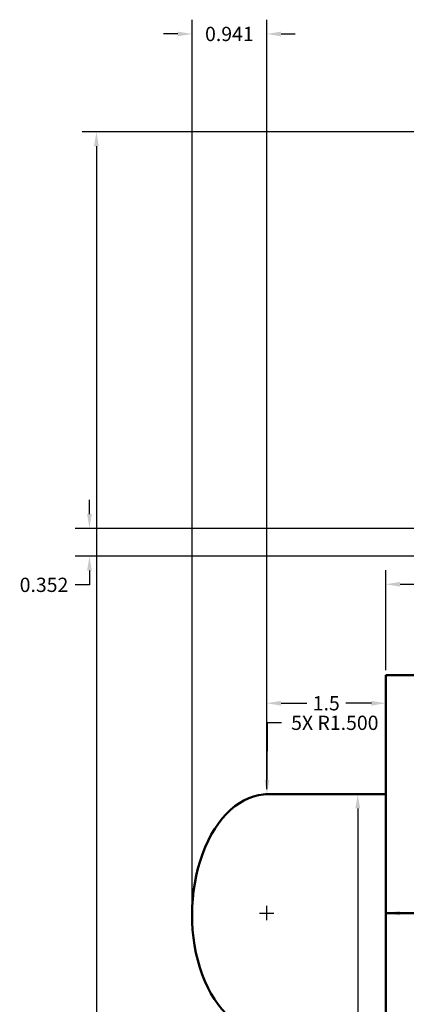
# Model space of a CAD drawing. Units: inches. Extents: x 15.4 to 41.1, y -0.4 to 25.1.
# Tile 2 of 4: x 15.4 to 20.3, y 12.7 to 25.1. Entities that reach past the tile are written whole.
import ezdxf

# ---------------------------------------------------------------- set-up
doc = ezdxf.new("R2010")
doc.units = ezdxf.units.IN
doc.header["$MEASUREMENT"] = 0
doc.layers.add('M-DIMS', color=2, linetype='Continuous', lineweight=18)
doc.layers.add('M-OUTL', color=7, linetype='Continuous', lineweight=50)
doc.styles.get("Standard").update_dxf_attribs({"font": 'arial.ttf'})
doc.dimstyles.get("Standard").update_dxf_attribs({"dimtxt": 0.18, "dimasz": 0.18, "dimexe": 0.18, "dimexo": 0.0625, "dimgap": 0.09, "dimtad": 0, "dimtih": 1, "dimtoh": 1, "dimdec": 4, "dimzin": 0, "dimdsep": 46, "dimtxsty": 'Standard', "dimcen": 0.09, "dimadec": 0, "dimazin": 0, "dimtfac": 1, "dimtdec": 4, "dimtofl": 0, "dimtmove": 0, "dimatfit": 3, "dimfxl": 1, "dimtolj": 1, "dimtzin": 0, "dimarcsym": 0})

# ---------------------------------------------------------------- blocks, each defined once
blk = doc.blocks.new('*D2')
at = {"layer": 'Defpoints', "color": 0, "transparency": 16777216}
for p in [(16.366, 23.727), (20.763, 23.727), (20.763, 1.022)]:
    blk.add_point(p, dxfattribs=at)
at = {"layer": 'M-DIMS', "color": 0, "lineweight": -2, "transparency": 16777216}
for p, q in [((20.7, 23.727), (16.186, 23.727)), ((16.366, 23.547), (16.366, 12.557)), ((16.366, 1.202), (16.366, 12.193)), ((20.7, 1.022), (16.186, 1.022))]:
    blk.add_line(p, q, dxfattribs=at)
at = {"layer": 'M-DIMS', "color": 0, "transparency": 16777216}
for points in [[(16.336, 23.547), (16.396, 23.547), (16.366, 23.727)], [(16.336, 1.202), (16.396, 1.202), (16.366, 1.022)]]:
    blk.add_solid(points, dxfattribs=at)
at = {"layer": 'M-DIMS', "color": 0, "transparency": 16777216, "insert": (16.366, 12.375), "char_height": 0.18, "attachment_point": 5}
blk.add_mtext('\\A1;22.705', dxfattribs=at)
blk = doc.blocks.new('*D20')
at = {"layer": 'Defpoints', "color": 0, "transparency": 16777216}
for p in [(21.513, 18.022), (20.013, 16.875), (21.513, 16.875)]:
    blk.add_point(p, dxfattribs=at)
at = {"layer": 'M-DIMS', "color": 0, "lineweight": -2, "transparency": 16777216}
for p, q in [((20.013, 16.937), (20.013, 18.202)), ((21.513, 16.937), (21.513, 18.202)), ((20.193, 18.022), (20.517, 18.022)), ((21.333, 18.022), (21.009, 18.022))]:
    blk.add_line(p, q, dxfattribs=at)
at = {"layer": 'M-DIMS', "color": 0, "transparency": 16777216}
for points in [[(20.193, 18.052), (20.193, 17.992), (20.013, 18.022)], [(21.333, 18.052), (21.333, 17.992), (21.513, 18.022)]]:
    blk.add_solid(points, dxfattribs=at)
at = {"layer": 'M-DIMS', "color": 0, "transparency": 16777216, "insert": (20.763, 18.022), "char_height": 0.18, "attachment_point": 5}
blk.add_mtext('\\A1;1.5', dxfattribs=at)
blk = doc.blocks.new('*D21')
at = {"layer": 'Defpoints', "color": 0, "transparency": 16777216}
for p in [(20.013, 16.875), (20.013, 7.875), (21.16, 7.875)]:
    blk.add_point(p, dxfattribs=at)
at = {"layer": 'M-DIMS', "color": 0, "lineweight": -2, "transparency": 16777216}
for p, q in [((20.075, 16.875), (21.34, 16.875)), ((21.16, 16.695), (21.16, 12.557)), ((21.16, 8.055), (21.16, 12.193)), ((20.075, 7.875), (21.34, 7.875))]:
    blk.add_line(p, q, dxfattribs=at)
at = {"layer": 'M-DIMS', "color": 0, "transparency": 16777216}
for points in [[(21.13, 16.695), (21.19, 16.695), (21.16, 16.875)], [(21.13, 8.055), (21.19, 8.055), (21.16, 7.875)]]:
    blk.add_solid(points, dxfattribs=at)
at = {"layer": 'M-DIMS', "color": 0, "transparency": 16777216, "insert": (21.16, 12.375), "char_height": 0.18, "attachment_point": 5}
blk.add_mtext('\\A1;9', dxfattribs=at)
blk = doc.blocks.new('*D22')
at = {"layer": 'Defpoints', "color": 0, "transparency": 16777216}
for p in [(20.013, 16.522), (18.513, 15.375), (20.013, 15.375)]:
    blk.add_point(p, dxfattribs=at)
at = {"layer": 'M-DIMS', "color": 0, "lineweight": -2, "transparency": 16777216}
for p, q in [((18.513, 15.437), (18.513, 16.702)), ((20.013, 15.437), (20.013, 16.702)), ((18.693, 16.522), (19.017, 16.522)), ((19.833, 16.522), (19.509, 16.522))]:
    blk.add_line(p, q, dxfattribs=at)
at = {"layer": 'M-DIMS', "color": 0, "transparency": 16777216}
for points in [[(18.693, 16.552), (18.693, 16.492), (18.513, 16.522)], [(19.833, 16.552), (19.833, 16.492), (20.013, 16.522)]]:
    blk.add_solid(points, dxfattribs=at)
at = {"layer": 'M-DIMS', "color": 0, "transparency": 16777216, "insert": (19.263, 16.522), "char_height": 0.18, "attachment_point": 5}
blk.add_mtext('\\A1;1.5', dxfattribs=at)
blk = doc.blocks.new('*D23')
at = {"layer": 'Defpoints', "color": 0, "transparency": 16777216}
for p in [(18.513, 15.375), (18.518, 9.375), (19.665, 9.376)]:
    blk.add_point(p, dxfattribs=at)
at = {"layer": 'M-DIMS', "color": 0, "lineweight": -2, "transparency": 16777216}
for p, q in [((18.575, 15.375), (19.84, 15.376)), ((19.66, 15.196), (19.663, 12.558)), ((19.665, 9.556), (19.663, 12.194)), ((18.58, 9.375), (19.845, 9.376))]:
    blk.add_line(p, q, dxfattribs=at)
at = {"layer": 'M-DIMS', "color": 0, "transparency": 16777216}
for points in [[(19.69, 15.196), (19.63, 15.196), (19.66, 15.376)], [(19.695, 9.556), (19.635, 9.556), (19.665, 9.376)]]:
    blk.add_solid(points, dxfattribs=at)
at = {"layer": 'M-DIMS', "color": 0, "transparency": 16777216, "insert": (19.663, 12.376), "char_height": 0.18, "attachment_point": 5}
blk.add_mtext('\\A1;6', dxfattribs=at)
blk = doc.blocks.new('*D35')
at = {"layer": 'Defpoints', "color": 0, "transparency": 16777216}
for p in [(18.513, 13.875), (20.013, 13.875)]:
    blk.add_point(p, dxfattribs=at)
at = {"layer": 'M-DIMS', "color": 0, "lineweight": -2, "transparency": 16777216}
for p, q in [((18.513, 13.785), (18.513, 13.965)), ((18.423, 13.875), (18.603, 13.875)), ((20.913, 13.875), (20.193, 13.875))]:
    blk.add_line(p, q, dxfattribs=at)
at = {"layer": 'M-DIMS', "color": 0, "transparency": 16777216}
blk.add_solid([(20.193, 13.905), (20.193, 13.845), (20.013, 13.875)], dxfattribs=at)
at = {"layer": 'M-DIMS', "color": 0, "transparency": 16777216, "insert": (21.516, 13.875), "char_height": 0.18, "attachment_point": 5}
blk.add_mtext('\\A1;5X R1.50', dxfattribs=at)
blk = doc.blocks.new('*D42')
at = {"layer": 'Defpoints', "color": 0, "transparency": 16777216}
for p in [(23.368, 18.727), (16.278, 18.375), (23.013, 18.375)]:
    blk.add_point(p, dxfattribs=at)
at = {"layer": 'M-DIMS', "color": 0, "lineweight": -2, "transparency": 16777216}
for p, q in [((16.278, 18.907), (16.278, 19.087)), ((23.305, 18.727), (16.098, 18.727)), ((22.95, 18.375), (16.098, 18.375)), ((16.278, 18.195), (16.278, 18.015)), ((16.278, 18.015), (16.098, 18.015))]:
    blk.add_line(p, q, dxfattribs=at)
at = {"layer": 'M-DIMS', "color": 0, "transparency": 16777216}
for points in [[(16.248, 18.907), (16.308, 18.907), (16.278, 18.727)], [(16.248, 18.195), (16.308, 18.195), (16.278, 18.375)]]:
    blk.add_solid(points, dxfattribs=at)
at = {"layer": 'M-DIMS', "color": 0, "transparency": 16777216, "insert": (15.705, 18.015), "char_height": 0.18, "attachment_point": 5}
blk.add_mtext('\\A1;0.352', dxfattribs=at)
blk = doc.blocks.new('*D51')
at = {"layer": 'Defpoints', "color": 0, "transparency": 16777216}
for p in [(18.513, 24.962), (18.513, 15.375), (17.571, 13.858)]:
    blk.add_point(p, dxfattribs=at)
at = {"layer": 'M-DIMS', "color": 0, "lineweight": -2, "transparency": 16777216}
for p, q in [((17.571, 13.921), (17.571, 25.142)), ((18.513, 15.437), (18.513, 25.142)), ((17.391, 24.962), (17.211, 24.962)), ((18.693, 24.962), (18.873, 24.962))]:
    blk.add_line(p, q, dxfattribs=at)
at = {"layer": 'M-DIMS', "color": 0, "transparency": 16777216}
for points in [[(17.391, 24.992), (17.391, 24.932), (17.571, 24.962)], [(18.693, 24.992), (18.693, 24.932), (18.513, 24.962)]]:
    blk.add_solid(points, dxfattribs=at)
at = {"layer": 'M-DIMS', "color": 0, "transparency": 16777216, "insert": (18.042, 24.962), "char_height": 0.18, "attachment_point": 5}
blk.add_mtext('\\A1;0.941', dxfattribs=at)
blk = doc.blocks.new('*D55')
at = {"layer": 'Defpoints', "color": 0, "transparency": 16777216}
for p in [(18.516, 15.375), (18.513, 13.875)]:
    blk.add_point(p, dxfattribs=at)
at = {"layer": 'M-DIMS', "color": 0, "lineweight": -2, "transparency": 16777216}
for p, q in [((18.518, 16.275), (18.516, 15.555)), ((18.698, 16.275), (18.518, 16.275)), ((18.513, 13.785), (18.513, 13.965)), ((18.423, 13.875), (18.603, 13.875))]:
    blk.add_line(p, q, dxfattribs=at)
at = {"layer": 'M-DIMS', "color": 0, "transparency": 16777216}
blk.add_solid([(18.486, 15.555), (18.546, 15.555), (18.516, 15.375)], dxfattribs=at)
at = {"layer": 'M-DIMS', "color": 0, "transparency": 16777216, "insert": (19.371, 16.275), "char_height": 0.18, "attachment_point": 5}
blk.add_mtext('\\A1;5X R1.500', dxfattribs=at)

msp = doc.modelspace()

# ---------------------------------------------------------------- linework, layer by layer
at = {"layer": 'M-OUTL'}
for p, q in [((20.0128, 13.8747), (20.0128, 16.8747)), ((20.0128, 16.8747), (21.0128, 16.8747)), ((18.4971, 15.374), (18.4971, 15.3748)), ((20.0128, 15.3747), (18.5128, 15.3747)), ((20.0128, 12.3747), (20.0128, 13.8747)), ((20.0128, 13.8747), (24.0128, 13.8747)), ((24.0128, 13.8747), (20.0128, 13.8747))]:
    msp.add_line(p, q, dxfattribs=at)
for start, end in [(89.15251, 90.60328), (358.88885, 1.11115)]:
    msp.add_arc((18.5129, 13.8747), 1.5002, start, end, dxfattribs=at)
msp.add_ellipse((18.5129, 13.8747), major_axis=(0.0222, 1.5), ratio=0.6275384, start_param=0, end_param=3.1819287, dxfattribs=at)

# ---------------------------------------------------------------- dimensions: what is measured, and where the dimension line sits
at = {"layer": 'M-DIMS'}
for base, p1, p2, override, picture, middle in [((18.51279, 24.96201), (17.57133, 13.85835), (18.51279, 15.37469), {"dimdec": 3, "dimlfac": 1, "dimrnd": 0, "dimzin": 0, "dimdsep": 46, "dimlunit": 2}, '*D51', (18.04206, 24.96201)), ((21.5128, 18.0222), (20.0128, 16.8747), (21.5128, 16.8747), {"dimdec": 1, "dimlfac": 1, "dimrnd": 0, "dimzin": 0, "dimdsep": 46, "dimlunit": 2}, '*D20', (20.7628, 18.0222)), ((20.0128, 16.5222), (18.5128, 15.3747), (20.0128, 15.3747), {"dimdec": 1, "dimlfac": 1, "dimrnd": 0, "dimzin": 0, "dimdsep": 46, "dimlunit": 2}, '*D22', (19.2628, 16.5222))]:
    dim = msp.add_linear_dim(base=base, p1=p1, p2=p2, dimstyle='Standard', override=override, dxfattribs=at)
    dim.commit()
    dim.dimension.update_dxf_attribs({"geometry": picture, "text_midpoint": middle})
for base, p1, p2, angle, override, picture, middle in [((16.3657, 23.727), (20.7628, 1.0224), (20.7628, 23.727), 90, {"dimdec": 3, "dimlfac": 1, "dimrnd": 0, "dimzin": 0, "dimdsep": 46, "dimlunit": 2}, '*D2', (16.3657, 12.3747)), ((16.2782, 18.3747), (23.3676, 18.727), (23.0128, 18.3747), 90, {"dimdec": 3, "dimlfac": 1, "dimrnd": 0, "dimzin": 0, "dimdsep": 46, "dimlunit": 2}, '*D42', (15.7054, 18.0147)), ((21.1603, 7.8747), (20.0128, 16.8747), (20.0128, 7.8747), 270, {"dimdec": 0, "dimlfac": 1, "dimrnd": 0, "dimzin": 0, "dimdsep": 46, "dimlunit": 2}, '*D21', (21.1603, 12.3747)), ((19.6655, 9.3757), (18.5128, 15.3747), (18.518, 9.3747), 270.0497, {"dimdec": 0, "dimlfac": 1, "dimrnd": 0, "dimzin": 0, "dimdsep": 46, "dimlunit": 2}, '*D23', (19.6629, 12.3757))]:
    dim = msp.add_linear_dim(base=base, p1=p1, p2=p2, angle=angle, dimstyle='Standard', override=override, dxfattribs=at)
    dim.commit()
    dim.dimension.update_dxf_attribs({"geometry": picture, "text_midpoint": middle})
for mpoint, override, picture, middle in [((18.516, 15.3749), {"dimdec": 3, "dimlfac": 1, "dimrnd": 0, "dimzin": 0, "dimdsep": 46, "dimlunit": 2}, '*D55', (19.3708, 16.275)), ((20.0131, 13.875), {"dimdec": 2, "dimlfac": 1, "dimrnd": 0, "dimzin": 0, "dimdsep": 46, "dimlunit": 2}, '*D35', (20.9132, 13.8752))]:
    dim = msp.add_radius_dim(center=(18.5129, 13.8747), mpoint=mpoint, text='5X <>', dimstyle='Standard', override=override, dxfattribs=at)
    dim.commit()
    dim.dimension.update_dxf_attribs({"geometry": picture, "text_midpoint": middle, "dimtype": 164})

doc.saveas('drawing.dxf')
